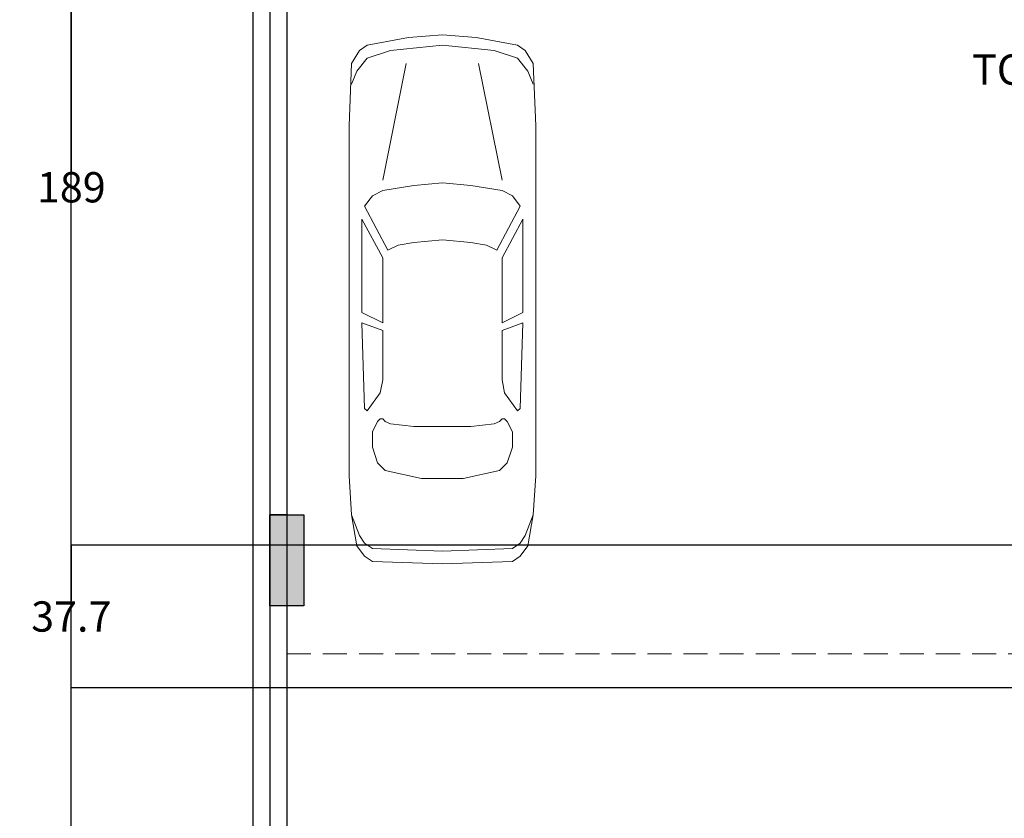
# Model space of a CAD drawing. Units: inches. Extents: x -48 to 50072, y 0 to 21068.
# Tile 45 of 75: x -48 to 212, y 417 to 628. Entities that reach past the tile are written whole.
import ezdxf

# ---------------------------------------------------------------- set-up
doc = ezdxf.new("R2010")
doc.units = ezdxf.units.IN
doc.header["$MEASUREMENT"] = 0
doc.linetypes.add('ACAD_ISO02W100', pattern=[15, 12, -3])
doc.linetypes.add('HIDDEN', pattern=[9.525, 6.35, -3.175])
for name, color, linetype, lineweight in [('A-ANNO-DIMS', 2, 'Continuous', 18), ('A-COLS', 1, 'Continuous', 35), ('A-FLOR-OVHD', 8, 'HIDDEN', 13), ('A-WALL', 7, 'Continuous', 35), ('C-PROP', 7, 'Continuous', 25), ('C-PROP-REF', 32, 'ACAD_ISO02W100', 13), ('C-SITE-VEHC', 8, 'Continuous', 13)]:
    doc.layers.add(name, color=color, linetype=linetype, lineweight=lineweight)
doc.styles.get("Standard").update_dxf_attribs({"font": 'arial.ttf'})
doc.dimstyles.get("Standard").update_dxf_attribs({"dimtxt": 8, "dimasz": 0.18, "dimexe": 0.18, "dimexo": 0.0625, "dimgap": 0.09, "dimtad": 0, "dimtih": 1, "dimtoh": 1, "dimdec": 1, "dimzin": 0, "dimdsep": 46, "dimlunit": 4, "dimtxsty": 'Standard', "dimblk": 'ARCHTICK', "dimcen": 0.09, "dimadec": 0, "dimazin": 0, "dimtfac": 1, "dimtdec": 1, "dimtofl": 0, "dimtmove": 0, "dimatfit": 3, "dimldrblk": 'ARCHTICK', "dimfxl": 1, "dimtolj": 1, "dimtzin": 0, "dimarcsym": 0})

# ---------------------------------------------------------------- blocks, each defined once
blk = doc.blocks.new('bnniku')
at = {"layer": 'Defpoints'}
h = blk.add_hatch(color=256, dxfattribs=at)
h.dxf.hatch_style = 1
h.paths.add_polyline_path([(767.55, 1114.04), (758.55, 1114.04), (758.55, 1090.04), (767.55, 1090.04)])
for p, q in [((758.55, 1114.04), (767.55, 1114.04)), ((758.55, 1090.04), (758.55, 1114.04)), ((767.55, 1114.04), (767.55, 1090.04)), ((767.55, 1090.04), (758.55, 1090.04))]:
    blk.add_line(p, q, dxfattribs=at)
blk = doc.blocks.new('CAR-PLAN-SEDAN')
for p, q in [((15.75, 139.03), (4.79, 136.97)), ((24.65, 139.71), (15.75, 139.03)), ((24.65, 139.71), (33.56, 139.03)), ((33.56, 139.03), (44.52, 136.97)), ((2.74, 135.6), (0.68, 132.18)), ((4.79, 136.97), (2.74, 135.6)), ((10.96, 135.6), (4.79, 133.55)), ((24.65, 136.97), (10.96, 135.6)), ((24.65, 136.97), (38.35, 135.6)), ((38.35, 135.6), (44.52, 133.55)), ((44.52, 136.97), (46.57, 135.6)), ((46.57, 135.6), (48.62, 132.18)), ((4.79, 133.55), (2.05, 130.12)), ((44.52, 133.55), (47.25, 130.12)), ((0.68, 132.18), (0, 115.74)), ((2.05, 130.12), (0.68, 126.7)), ((15.07, 132.18), (8.9, 101.36)), ((34.24, 132.18), (40.41, 101.36)), ((47.25, 130.12), (48.62, 126.7)), ((48.62, 132.18), (49.31, 115.74)), ((0, 115.74), (0, 23.29)), ((49.31, 115.74), (49.31, 23.29)), ((17.12, 99.99), (8.9, 98.62)), ((24.65, 100.67), (17.12, 99.99)), ((24.65, 100.67), (32.19, 99.99)), ((32.19, 99.99), (40.41, 98.62)), ((6.16, 97.25), (4.11, 94.51)), ((8.9, 98.62), (6.16, 97.25)), ((40.41, 98.62), (43.15, 97.25)), ((43.15, 97.25), (45.2, 94.51)), ((4.11, 94.51), (10.27, 82.87)), ((45.2, 94.51), (39.04, 82.87)), ((3.42, 91.09), (8.9, 80.81)), ((3.42, 66.43), (3.42, 91.09)), ((45.88, 91.09), (40.41, 80.81)), ((45.88, 66.43), (45.88, 91.09)), ((10.27, 82.87), (13.01, 84.24)), ((13.01, 84.24), (17.12, 84.92)), ((17.12, 84.92), (24.65, 85.61)), ((32.19, 84.92), (24.65, 85.61)), ((36.3, 84.24), (32.19, 84.92)), ((39.04, 82.87), (36.3, 84.24)), ((8.9, 80.81), (8.9, 63.69)), ((40.41, 80.81), (40.41, 63.69)), ((8.9, 63.69), (3.42, 66.43)), ((40.41, 63.69), (45.88, 66.43)), ((4.11, 41.09), (3.42, 63.69)), ((3.42, 63.69), (8.9, 61.64)), ((45.88, 63.69), (40.41, 61.64)), ((45.2, 41.09), (45.88, 63.69)), ((8.9, 61.64), (8.9, 48.62)), ((40.41, 61.64), (40.41, 48.62)), ((8.9, 48.62), (8.22, 45.2)), ((40.41, 48.62), (41.09, 45.2)), ((8.22, 45.2), (4.79, 40.41)), ((41.09, 45.2), (44.52, 40.41)), ((4.79, 40.41), (4.11, 41.09)), ((44.52, 40.41), (45.2, 41.09)), ((7.53, 37.67), (6.16, 34.93)), ((8.22, 38.35), (7.53, 37.67)), ((8.9, 38.35), (8.22, 38.35)), ((9.59, 37.67), (8.9, 38.35)), ((10.96, 36.98), (9.59, 37.67)), ((17.12, 36.3), (10.96, 36.98)), ((32.19, 36.3), (38.35, 36.98)), ((38.35, 36.98), (39.72, 37.67)), ((39.72, 37.67), (40.41, 38.35)), ((40.41, 38.35), (41.09, 38.35)), ((41.09, 38.35), (41.78, 37.67)), ((41.78, 37.67), (43.15, 34.93)), ((6.16, 34.93), (6.16, 30.82)), ((24.65, 36.3), (17.12, 36.3)), ((24.65, 36.3), (32.19, 36.3)), ((43.15, 34.93), (43.15, 30.82)), ((6.16, 30.82), (7.53, 26.71)), ((43.15, 30.82), (41.78, 26.71)), ((7.53, 26.71), (9.59, 24.65)), ((41.78, 26.71), (39.72, 24.65)), ((9.59, 24.65), (19.18, 22.6)), ((39.72, 24.65), (30.13, 22.6)), ((0, 23.29), (0.68, 13.01)), ((19.18, 22.6), (24.65, 22.6)), ((30.13, 22.6), (24.65, 22.6)), ((49.31, 23.29), (48.62, 13.01)), ((0.68, 13.01), (2.74, 7.53)), ((0.68, 13.01), (2.05, 4.79)), ((48.62, 13.01), (46.57, 7.53)), ((48.62, 13.01), (47.25, 4.79)), ((2.74, 7.53), (4.11, 5.48)), ((4.11, 5.48), (6.16, 4.11)), ((45.2, 5.48), (43.15, 4.11)), ((46.57, 7.53), (45.2, 5.48)), ((2.05, 4.79), (4.11, 2.05)), ((6.16, 4.11), (24.65, 3.42)), ((43.15, 4.11), (24.65, 3.42)), ((47.25, 4.79), (45.2, 2.05)), ((4.11, 2.05), (6.16, 0.69)), ((6.16, 0.69), (24.65, 0)), ((43.15, 0.69), (24.65, 0)), ((45.2, 2.05), (43.15, 0.69))]:
    blk.add_line(p, q)
blk = doc.blocks.new('_ArchTick')
at = {"color": 0, "linetype": 'ByBlock', "const_width": 0.15}
blk.add_lwpolyline([(-0.5, -0.5), (0.5, 0.5)], dxfattribs=at)
blk = doc.blocks.new('*D68')
at = {"layer": 'A-ANNO-DIMS', "color": 0, "lineweight": -2, "transparency": 16777216}
for p, q in [((257.08, 632.91), (262.77, 632.91)), ((262.59, 632.91), (262.59, 618.57)), ((262.59, 595.77), (262.59, 610.11)), ((257.08, 595.77), (262.77, 595.77))]:
    blk.add_line(p, q, dxfattribs=at)
at = {"layer": 'Defpoints', "color": 0, "transparency": 16777216}
for p in [(257.02, 632.91), (257.02, 595.77), (262.59, 595.77)]:
    blk.add_point(p, dxfattribs=at)
at = {"layer": 'A-ANNO-DIMS', "color": 0, "lineweight": -2, "transparency": 16777216, "xscale": 0.18, "yscale": 0.18, "zscale": 0.18}
for p, rotation in [((262.59, 632.91), 90), ((262.59, 595.77), 270)]:
    blk.add_blockref('_ArchTick', p, dxfattribs=dict(at, rotation=rotation))
at = {"layer": 'A-ANNO-DIMS', "color": 0, "transparency": 16777216, "insert": (262.59, 614.34), "char_height": 8, "attachment_point": 5}
blk.add_mtext('\\A1;TOILET DOOR A 37 TYP.', dxfattribs=at)
blk = doc.blocks.new('*D113')
at = {"layer": 'A-ANNO-DIMS', "color": 0, "lineweight": -2, "transparency": 16777216}
for p, q in [((13.45, 1170.77), (-34.61, 1170.77)), ((-34.43, 1170.77), (-34.43, 696.6)), ((-34.43, 214.07), (-34.43, 688.25)), ((13.45, 214.07), (-34.61, 214.07))]:
    blk.add_line(p, q, dxfattribs=at)
at = {"layer": 'Defpoints', "color": 0, "transparency": 16777216}
for p in [(-34.43, 1170.77), (13.52, 1170.77), (13.52, 214.07)]:
    blk.add_point(p, dxfattribs=at)
at = {"layer": 'A-ANNO-DIMS', "color": 0, "lineweight": -2, "transparency": 16777216, "xscale": 0.18, "yscale": 0.18, "zscale": 0.18}
for p, rotation in [((-34.43, 1170.77), 90), ((-34.43, 214.07), 270)]:
    blk.add_blockref('_ArchTick', p, dxfattribs=dict(at, rotation=rotation))
at = {"layer": 'A-ANNO-DIMS', "color": 0, "transparency": 16777216, "insert": (-34.43, 692.42), "char_height": 8, "attachment_point": 5}
blk.add_mtext('\\A1;956.7', dxfattribs=at)
blk = doc.blocks.new('*D116')
at = {"layer": 'A-ANNO-DIMS', "color": 0, "lineweight": -2, "transparency": 16777216}
for p, q in [((18.02, 677.71), (18.02, 165.94)), ((216.02, 677.71), (216.02, 165.94)), ((18.02, 166.12), (108.46, 166.12)), ((216.02, 166.12), (125.58, 166.12))]:
    blk.add_line(p, q, dxfattribs=at)
at = {"layer": 'Defpoints', "color": 0, "transparency": 16777216}
for p in [(18.02, 677.77), (216.02, 677.77), (216.02, 166.12)]:
    blk.add_point(p, dxfattribs=at)
at = {"layer": 'A-ANNO-DIMS', "color": 0, "lineweight": -2, "transparency": 16777216, "xscale": 0.18, "yscale": 0.18, "zscale": 0.18, "rotation": 180}
blk.add_blockref('_ArchTick', (18.02, 166.12), dxfattribs=at)
at = {"layer": 'A-ANNO-DIMS', "color": 0, "lineweight": -2, "transparency": 16777216, "xscale": 0.18, "yscale": 0.18, "zscale": 0.18}
blk.add_blockref('_ArchTick', (216.02, 166.12), dxfattribs=at)
at = {"layer": 'A-ANNO-DIMS', "color": 0, "transparency": 16777216, "insert": (117.02, 166.12), "char_height": 8, "attachment_point": 5}
blk.add_mtext('\\A1;198', dxfattribs=at)
blk = doc.blocks.new('*D127')
at = {"layer": 'A-ANNO-DIMS', "color": 0, "lineweight": -2, "transparency": 16777216}
for p, q in [((215.95, 677.77), (-34.61, 677.77)), ((-34.43, 677.77), (-34.43, 587.45)), ((-34.43, 488.77), (-34.43, 579.1)), ((215.95, 488.77), (-34.61, 488.77))]:
    blk.add_line(p, q, dxfattribs=at)
at = {"layer": 'Defpoints', "color": 0, "transparency": 16777216}
for p in [(-34.43, 677.77), (216.02, 677.77), (216.02, 488.77)]:
    blk.add_point(p, dxfattribs=at)
at = {"layer": 'A-ANNO-DIMS', "color": 0, "lineweight": -2, "transparency": 16777216, "xscale": 0.18, "yscale": 0.18, "zscale": 0.18}
for p, rotation in [((-34.43, 677.77), 90), ((-34.43, 488.77), 270)]:
    blk.add_blockref('_ArchTick', p, dxfattribs=dict(at, rotation=rotation))
at = {"layer": 'A-ANNO-DIMS', "color": 0, "transparency": 16777216, "insert": (-34.43, 583.27), "char_height": 8, "attachment_point": 5}
blk.add_mtext('\\A1;189', dxfattribs=at)
blk = doc.blocks.new('*D128')
at = {"layer": 'A-ANNO-DIMS', "color": 0, "lineweight": -2, "transparency": 16777216}
for p, q in [((463.45, 488.77), (-34.61, 488.77)), ((-34.43, 488.77), (-34.43, 474.1)), ((-34.43, 451.07), (-34.43, 465.75)), ((463.45, 451.07), (-34.61, 451.07))]:
    blk.add_line(p, q, dxfattribs=at)
at = {"layer": 'Defpoints', "color": 0, "transparency": 16777216}
for p in [(-34.43, 488.77), (463.52, 488.77), (463.52, 451.07)]:
    blk.add_point(p, dxfattribs=at)
at = {"layer": 'A-ANNO-DIMS', "color": 0, "lineweight": -2, "transparency": 16777216, "xscale": 0.18, "yscale": 0.18, "zscale": 0.18}
for p, rotation in [((-34.43, 488.77), 90), ((-34.43, 451.07), 270)]:
    blk.add_blockref('_ArchTick', p, dxfattribs=dict(at, rotation=rotation))
at = {"layer": 'A-ANNO-DIMS', "color": 0, "transparency": 16777216, "insert": (-34.43, 469.92), "char_height": 8, "attachment_point": 5}
blk.add_mtext('\\A1;37.7', dxfattribs=at)

msp = doc.modelspace()

# ---------------------------------------------------------------- linework, layer by layer
at = {"layer": 'A-FLOR-OVHD'}
msp.add_line((22.517, 460.075), (216.017, 460.075), dxfattribs=at)
at = {"layer": 'A-WALL'}
msp.add_line((18.017, 496.758), (22.517, 496.758), dxfattribs=at)
at = {"layer": 'C-PROP'}
for p, q in [((13.517, 1170.775), (13.517, 214.075)), ((22.517, 860.775), (22.517, 223.075))]:
    msp.add_line(p, q, dxfattribs=at)
at = {"layer": 'C-PROP-REF'}
msp.add_line((18.017, 1166.275), (18.017, 214.075), dxfattribs=at)

# ---------------------------------------------------------------- block references
at = {"layer": 'A-COLS'}
msp.add_blockref('bnniku', (-740.534, -617.279), dxfattribs=at)
at = {"layer": 'C-SITE-VEHC'}
msp.add_blockref('CAR-PLAN-SEDAN', (38.926, 483.784), dxfattribs=at)

# ---------------------------------------------------------------- dimensions: what is measured, and where the dimension line sits
at = {"layer": 'A-ANNO-DIMS'}
for base, p1, p2, override, picture, middle in [((-34.433, 1170.775), (13.517, 214.075), (13.517, 1170.775), {"dimdec": 1, "dimlfac": 1, "dimrnd": 0, "dimzin": 0, "dimdsep": 46, "dimlunit": 2}, '*D113', (-34.433, 692.425)), ((-34.433, 677.775), (216.017, 488.775), (216.017, 677.775), {"dimdec": 0, "dimlfac": 1, "dimrnd": 0, "dimzin": 0, "dimdsep": 46, "dimlunit": 2}, '*D127', (-34.433, 583.275)), ((-34.433, 488.775), (463.517, 451.075), (463.517, 488.775), {"dimdec": 1, "dimlfac": 1, "dimrnd": 0, "dimzin": 0, "dimdsep": 46, "dimlunit": 2}, '*D128', (-34.433, 469.925))]:
    dim = msp.add_linear_dim(base=base, p1=p1, p2=p2, angle=90, dimstyle='Standard', override=override, dxfattribs=at)
    dim.commit()
    dim.dimension.update_dxf_attribs({"geometry": picture, "text_midpoint": middle})
dim = msp.add_linear_dim(base=(216.017, 166.125), p1=(18.017, 677.775), p2=(216.017, 677.775), dimstyle='Standard', override={"dimdec": 0, "dimlfac": 1, "dimrnd": 0, "dimzin": 0, "dimdsep": 46, "dimlunit": 2}, dxfattribs=at)
dim.commit()
dim.dimension.update_dxf_attribs({"geometry": '*D116', "text_midpoint": (117.017, 166.125)})
dim = msp.add_linear_dim(base=(262.588, 595.775), p1=(257.017, 632.911), p2=(257.017, 595.775), angle=270, text='TOILET DOOR A <> TYP.', dimstyle='Standard', override={"dimdec": 0, "dimlfac": 1, "dimrnd": 0, "dimzin": 0, "dimdsep": 46, "dimlunit": 2}, dxfattribs=at)
dim.commit()
dim.dimension.update_dxf_attribs({"geometry": '*D68', "text_midpoint": (262.588, 614.343)})

doc.saveas('drawing.dxf')
